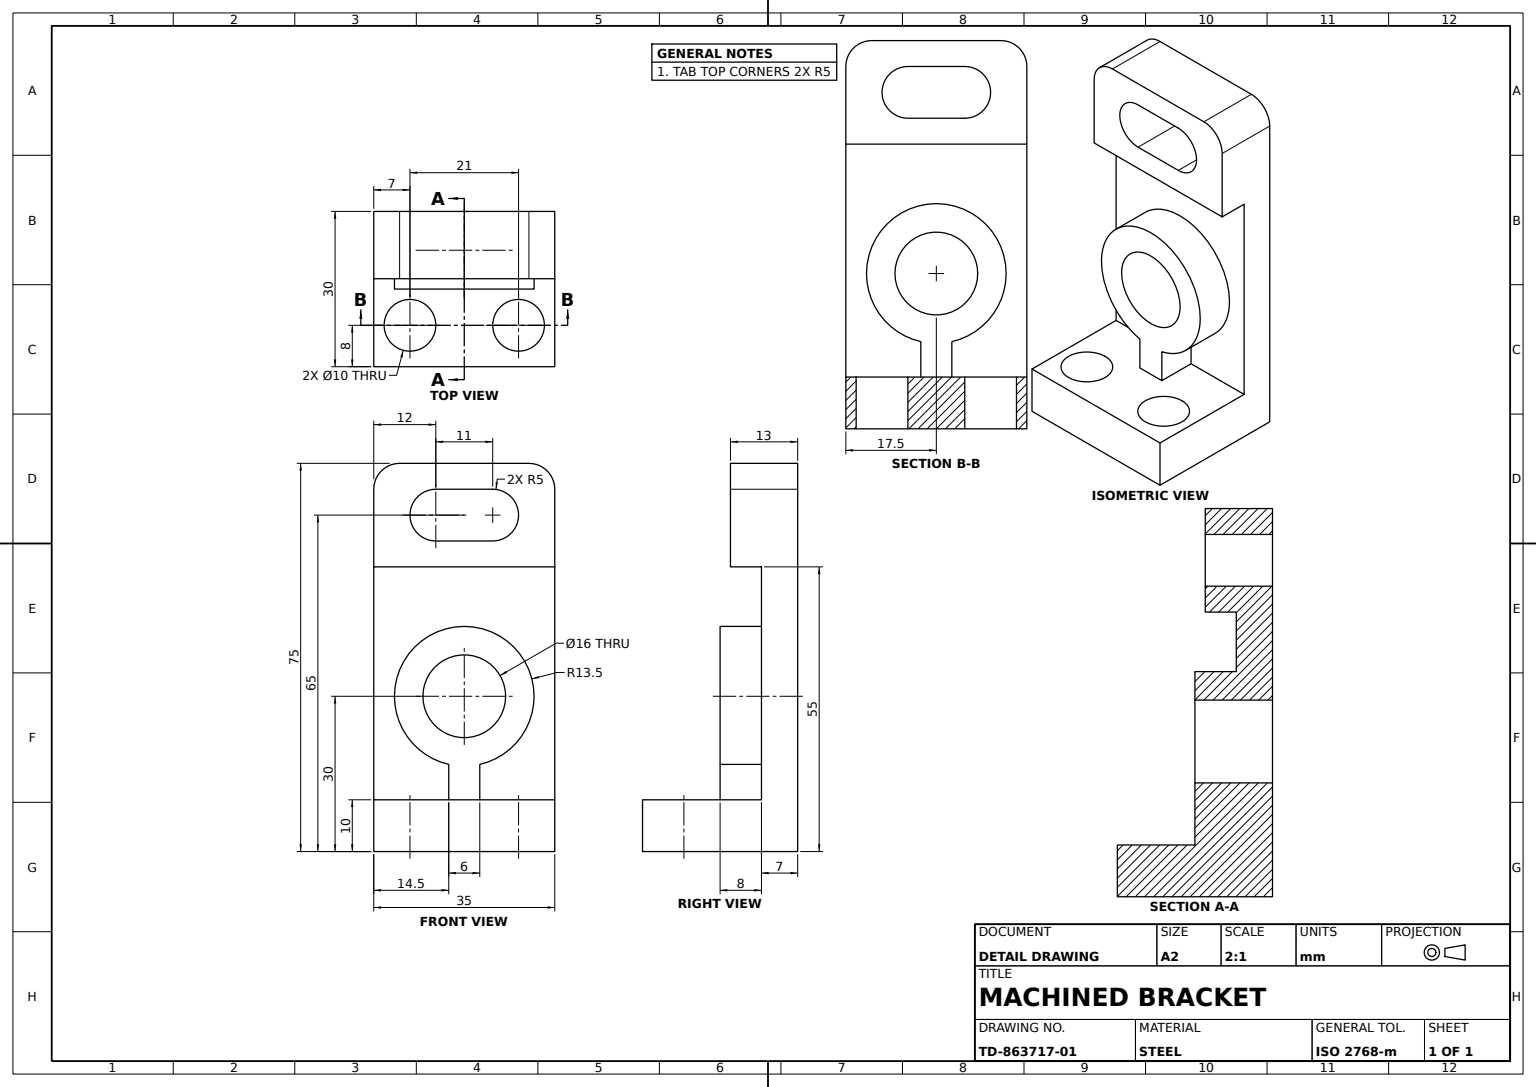
from build123d import *

# Parameters (mm, degrees)
L_BRACKET_BODY_DEPTH        = 17.5
TOP_CORNER_FILLET_R5_R      = 5
BORE_BOSS_DEPTH             = 8
BORE_AND_SLOT_SKETCH_R      = 8
BORE_AND_TOP_SLOT_CUT_DEPTH = 15
BASE_HOLES_SKETCH_R         = 5
BASE_MOUNTING_HOLES_DEPTH   = 10


with BuildPart() as part:
    # L Profile Sketch → L Bracket Body (new, symmetric)
    with BuildSketch(Plane(origin=(0, 0, 0), x_dir=(0, 0, -1), z_dir=(1, 0, 0))):
        Polygon((0, 0), (-30, 0), (-30, 10), (-7, 10), (-7, 55), (-13, 55), (-13, 75), (0, 75), align=None)
    extrude(amount=L_BRACKET_BODY_DEPTH, both=True)

    # Top Corner Fillet R5
    top_corner_fillet_r5_edges = [part.edges().sort_by_distance(p)[0] for p in [
        (-17.5, 75, 6.5),
        (17.5, 75, 6.5),
    ]]
    fillet(top_corner_fillet_r5_edges, radius=TOP_CORNER_FILLET_R5_R)

    # Bore Boss Sketch → Bore Boss (add)
    with BuildSketch(Plane.XY.offset(7)):
        with BuildLine():
            Line((-3, 16.837553419), (-3, 10))
            Line((-3, 10), (3, 10))
            Line((3, 10), (3, 16.837553419))
            ThreePointArc((3, 16.837553419), (0, 43.5), (-3, 16.837553419))
        make_face()
    extrude(amount=BORE_BOSS_DEPTH)

    # Bore and Slot Sketch → Bore and Top Slot Cut (cut)
    with BuildSketch(Plane.XY.offset(15)):
        with Locations((0, 30)):
            Circle(BORE_AND_SLOT_SKETCH_R)
        with BuildLine():
            Line((-5.5, 70), (5.5, 70))
            ThreePointArc((5.5, 70), (10.5, 65), (5.5, 60))
            Line((5.5, 60), (-5.5, 60))
            ThreePointArc((-5.5, 60), (-10.5, 65), (-5.5, 70))
        make_face()
    extrude(amount=-BORE_AND_TOP_SLOT_CUT_DEPTH, mode=Mode.SUBTRACT)

    # Base Holes Sketch → Base Mounting Holes (cut)
    with BuildSketch(Plane(origin=(0, 10, 0), x_dir=(1, 0, 0), z_dir=(0, 1, 0))):
        with Locations(Location((-10.5, -22, 0), (0, 0, 270))):
            Circle(BASE_HOLES_SKETCH_R)
        with Locations(Location((10.5, -22, 0), (0, 0, 270))):
            Circle(BASE_HOLES_SKETCH_R)
    extrude(amount=-BASE_MOUNTING_HOLES_DEPTH, mode=Mode.SUBTRACT)


solid = part.part
